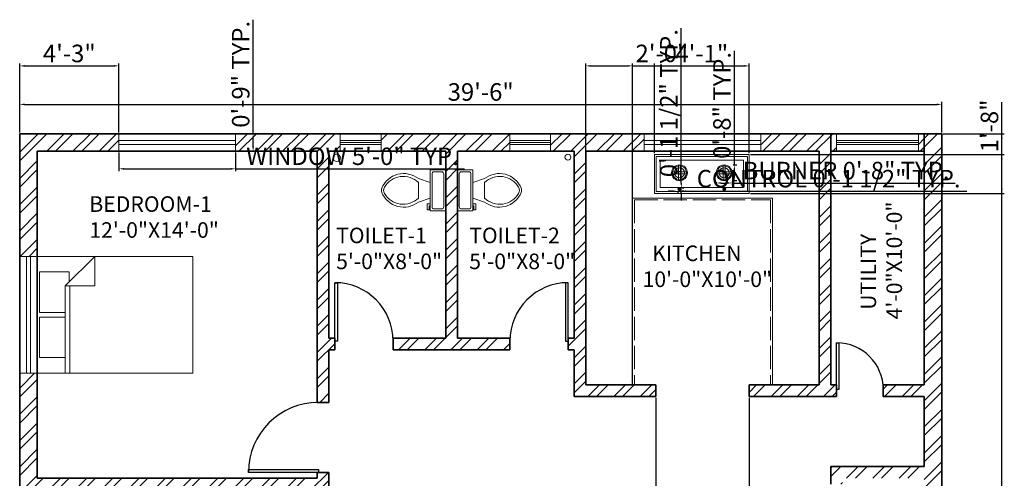
# Model space of a CAD drawing. Units: inches. Extents: x 600 to 1805, y 898 to 2057.
# Tile 3 of 5: x 642 to 1149, y 1822 to 2057. Entities that reach past the tile are written whole.
import ezdxf

# ---------------------------------------------------------------- set-up
doc = ezdxf.new("R2010")
doc.units = ezdxf.units.IN
doc.linetypes.add('ACAD_ISO02W100', pattern=[15, 12, -3])
for name, color, linetype, lineweight in [('A-ANNO-DIMS', 2, 'Continuous', 18), ('A-AREA-IDEN', 7, 'Continuous', 18), ('A-DOOR', 4, 'Continuous', 25), ('A-EQPM', 9, 'Continuous', 18), ('A-FLOR-CASE', 8, 'Continuous', 18), ('A-FLOR-CASE-HIDN', 8, 'ACAD_ISO02W100', 13), ('A-FLOR-FIXT', 8, 'Continuous', 18), ('A-FURN', 8, 'Continuous', 18), ('A-WALL', 7, 'Continuous', 35), ('A-WALL-PATT', 252, 'Continuous', 13)]:
    doc.layers.add(name, color=color, linetype=linetype, lineweight=lineweight)
doc.layers.add('A-GLAZ', color=244, linetype='Continuous', lineweight=20, true_color=0x991b1e)
doc.styles.get("Standard").update_dxf_attribs({"font": 'arial.ttf'})
doc.dimstyles.new('ISO-25', dxfattribs={"dimtxt": 9, "dimasz": 2.5, "dimexe": 1.25, "dimexo": 0.625, "dimtad": 1, "dimlunit": 3, "dimtxsty": 'Standard', "dimcen": 2.5, "dimadec": 0, "dimazin": 0, "dimtfac": 1, "dimtmove": 0, "dimatfit": 3, "dimfxl": 1, "dimarcsym": 0})

# ---------------------------------------------------------------- blocks, each defined once
blk = doc.blocks.new('*U2')
for p, q in [((0, 0), (0, -6)), ((40, 0), (40, -6))]:
    blk.add_line(p, q)
blk.add_lwpolyline([(0, 0), (0, 40), (1.75, 40), (1.75, 0)], close=True)
blk.add_arc((0, 0), 40, 0, 90)
blk = doc.blocks.new('*U3')
for p, q in [((0, 0), (0, -6)), ((-40, 0), (-40, -6))]:
    blk.add_line(p, q)
blk.add_lwpolyline([(0, 0), (0, 40), (-1.75, 40), (-1.75, 0)], close=True)
blk.add_arc((0, 0), 40, 90, 180)
blk = doc.blocks.new('*U4')
for p, q in [((0, 0), (0, -6)), ((40, 0), (40, -6))]:
    blk.add_line(p, q)
blk.add_lwpolyline([(0, 0), (0, 40), (1.75, 40), (1.75, 0)], close=True)
blk.add_arc((0, 0), 40, 0, 90)
blk = doc.blocks.new('Bed - Queen')
for p, q in [((0, -80.00003), (0, 0)), ((0, 0), (59.99999, 0)), ((59.99999, 0), (59.99999, -80.00003)), ((7.99999, -1.2), (28.79998, -1.2)), ((7.99999, -14.4), (7.99999, -1.2)), ((28.79998, -1.2), (28.79998, -14.4)), ((31.19999, -1.2), (51.99999, -1.2)), ((31.19999, -14.4), (31.19999, -1.2)), ((51.99999, -1.2), (51.99999, -16.4)), ((0, -14.4), (44.8, -14.4)), ((59.99999, -29.6), (44.8, -14.4)), ((44.8, -14.4), (44.8, -29.6)), ((44.8, -16.8), (0, -16.8)), ((51.99999, -16.4), (46.79936, -16.4)), ((44.8, -29.6), (59.99999, -29.6)), ((59.99999, -80.00003), (0, -80.00003))]:
    blk.add_line(p, q)
blk = doc.blocks.new('*U10')
for p, q in [((9.5, -6), (9.5, -2)), ((-10, -8.5), (-8, -8.5)), ((-10, -9.5), (-10, -8.5)), ((-7, -9.5), (-10, -9.5)), ((-8, -8.5), (-8, -8)), ((-7, -8), (-7, -9.5)), ((-4, -8), (-6, -14)), ((4, -8), (6, -14)), ((4, -14), (-4, -14))]:
    blk.add_line(p, q)
blk.add_lwpolyline([(10.5, -8), (10.5, 0), (-10.5, 0), (-10.5, -8)], close=True)
for points in [[(-9.5, -2), (-9.5, -6)], [(8.5, -1), (-8.5, -1)], [(-8.5, -7), (8.5, -7)]]:
    blk.add_lwpolyline(points)
for centre, radius, start, end in [((-8.62, -1.88), 0.884, 81.8699, 188.1301), ((8.62, -1.88), 0.884, 351.8699, 98.1301), ((-8.62, -6.12), 0.884, 171.8699, 278.1301), ((8.62, -6.12), 0.884, 261.8699, 8.1301), ((3.52, -21.58), 12.17, 141.4691, 247.9714), ((4.2, -21.82), 11.33, 136.3677, 238.9468), ((-3.52, -21.58), 12.17, 292.0284, 38.5307), ((-4.2, -21.82), 11.33, 301.053, 43.6321), ((0, -27.88), 4, 245.7318, 294.2682), ((0, -29), 4, 254.8605, 285.1395)]:
    blk.add_arc(centre, radius, start, end)
blk = doc.blocks.new('*D13')
at = {"layer": 'A-ANNO-DIMS', "color": 0, "lineweight": -2, "transparency": 16777216}
for p, q in [((642.39, 1999.48), (642.39, 2015.2)), ((1116.39, 1999.48), (1116.39, 2015.2)), ((644.89, 2013.95), (1113.89, 2013.95))]:
    blk.add_line(p, q, dxfattribs=at)
at = {"layer": 'A-ANNO-DIMS', "color": 0, "transparency": 16777216}
for points in [[(644.89, 2014.37), (644.89, 2013.53), (642.39, 2013.95)], [(1113.89, 2014.37), (1113.89, 2013.53), (1116.39, 2013.95)]]:
    blk.add_solid(points, dxfattribs=at)
at = {"layer": 'Defpoints', "color": 0, "transparency": 16777216}
for p in [(1116.39, 2013.95), (642.39, 1998.86), (1116.39, 1998.86)]:
    blk.add_point(p, dxfattribs=at)
at = {"layer": 'A-ANNO-DIMS', "color": 0, "transparency": 16777216, "insert": (879.39, 2019.17), "char_height": 9, "attachment_point": 5}
blk.add_mtext('39\'-6"', dxfattribs=at)
blk = doc.blocks.new('WIN-60x9')
for p, q in [((60, 5.5), (0, 5.5)), ((60, 3.5), (0, 3.5))]:
    blk.add_line(p, q)
blk.add_lwpolyline([(60, 0), (60, 9), (0, 9), (0, 0)], close=True)
blk = doc.blocks.new('VENT-21x9')
for p, q in [((0, 5.5), (21, 5.5)), ((0, 4.5), (21, 4.5)), ((0, 3.5), (21, 3.5))]:
    blk.add_line(p, q)
blk.add_lwpolyline([(21, 9), (21, 0), (0, 0), (0, 9)], close=True)
blk = doc.blocks.new('COOKTOP-BURNER')
for p, q in [((3.54, 8.05), (3.54, 0.03)), ((4.54, 8.05), (4.54, 0.03)), ((0.03, 4.54), (8.05, 4.54)), ((0.03, 3.54), (8.05, 3.54)), ((3.34, 4.74), (3.34, 3.34)), ((3.34, 4.74), (4.74, 4.74)), ((3.34, 3.34), (4.74, 3.34)), ((4.74, 4.74), (4.74, 3.34))]:
    blk.add_line(p, q)
for radius in [4.04, 3.54, 2.54]:
    blk.add_circle((4.04, 4.04), radius)
blk = doc.blocks.new('COOKTOP-CONTROL')
for p, q in [((0, 0.85), (1.49, 0.85)), ((0, 0.65), (1.49, 0.65))]:
    blk.add_line(p, q)
blk.add_circle((0.75, 0.75), 0.747)
for start, end in [(10.5316, 169.4684), (190.5316, 349.4684)]:
    blk.add_arc((0.75, 0.75), 0.547, start, end)
blk = doc.blocks.new('*D22')
at = {"layer": 'A-ANNO-DIMS', "color": 0, "lineweight": -2, "transparency": 16777216}
for p, q in [((693.39, 1989.23), (693.39, 1979.61)), ((753.39, 1989.23), (753.39, 1979.61)), ((695.89, 1980.86), (750.89, 1980.86)), ((753.39, 1980.86), (871.02, 1980.86))]:
    blk.add_line(p, q, dxfattribs=at)
at = {"layer": 'A-ANNO-DIMS', "color": 0, "transparency": 16777216}
for points in [[(695.89, 1981.28), (695.89, 1980.44), (693.39, 1980.86)], [(750.89, 1981.28), (750.89, 1980.44), (753.39, 1980.86)]]:
    blk.add_solid(points, dxfattribs=at)
at = {"layer": 'Defpoints', "color": 0, "transparency": 16777216}
for p in [(693.39, 1989.86), (753.39, 1989.86), (753.39, 1980.86)]:
    blk.add_point(p, dxfattribs=at)
at = {"layer": 'A-ANNO-DIMS', "color": 0, "transparency": 16777216, "insert": (813.46, 1986.14), "char_height": 9, "attachment_point": 5}
blk.add_mtext('WINDOW 5\'-0" TYP.', dxfattribs=at)
blk = doc.blocks.new('*D23')
at = {"layer": 'A-ANNO-DIMS', "color": 0, "lineweight": -2, "transparency": 16777216}
for p, q in [((762.39, 1998.86), (762.39, 2057.47)), ((754.01, 1998.86), (763.64, 1998.86)), ((762.39, 1992.36), (762.39, 1996.36)), ((754.01, 1989.86), (763.64, 1989.86))]:
    blk.add_line(p, q, dxfattribs=at)
at = {"layer": 'A-ANNO-DIMS', "color": 0, "transparency": 16777216}
for points in [[(761.97, 1996.36), (762.8, 1996.36), (762.39, 1998.86)], [(761.97, 1992.36), (762.8, 1992.36), (762.39, 1989.86)]]:
    blk.add_solid(points, dxfattribs=at)
at = {"layer": 'Defpoints', "color": 0, "transparency": 16777216}
for p in [(753.39, 1998.86), (762.39, 1998.86), (753.39, 1989.86)]:
    blk.add_point(p, dxfattribs=at)
at = {"layer": 'A-ANNO-DIMS', "color": 0, "transparency": 16777216, "insert": (757.17, 2029.41), "char_height": 9, "attachment_point": 5, "rotation": 90}
blk.add_mtext('0\'-9" TYP.', dxfattribs=at)
blk = doc.blocks.new('*D28')
at = {"layer": 'A-ANNO-DIMS', "color": 0, "lineweight": -2, "transparency": 16777216}
for p, q in [((1000.52, 1974.15), (1000.52, 1972.32)), ((1003.02, 1973.57), (1006.1, 1973.57)), ((1008.6, 1974.15), (1008.6, 1972.32)), ((1008.6, 1973.57), (1123.4, 1973.57))]:
    blk.add_line(p, q, dxfattribs=at)
at = {"layer": 'A-ANNO-DIMS', "color": 0, "transparency": 16777216}
for points in [[(1003.02, 1973.98), (1003.02, 1973.15), (1000.52, 1973.57)], [(1006.1, 1973.98), (1006.1, 1973.15), (1008.6, 1973.57)]]:
    blk.add_solid(points, dxfattribs=at)
at = {"layer": 'Defpoints', "color": 0, "transparency": 16777216}
for p in [(1000.52, 1974.78), (1008.6, 1974.78), (1008.6, 1973.57)]:
    blk.add_point(p, dxfattribs=at)
at = {"layer": 'A-ANNO-DIMS', "color": 0, "transparency": 16777216, "insert": (1067.25, 1978.79), "char_height": 9, "attachment_point": 5}
blk.add_mtext('BURNER 0\'-8" TYP.', dxfattribs=at)
blk = doc.blocks.new('*D29')
at = {"layer": 'A-ANNO-DIMS', "color": 0, "lineweight": -2, "transparency": 16777216}
for p, q in [((1009.81, 1982.86), (1009.81, 2041.47)), ((1009.23, 1982.86), (1011.06, 1982.86)), ((1009.81, 1977.28), (1009.81, 1980.36)), ((1009.23, 1974.78), (1011.06, 1974.78))]:
    blk.add_line(p, q, dxfattribs=at)
at = {"layer": 'A-ANNO-DIMS', "color": 0, "transparency": 16777216}
for points in [[(1009.4, 1980.36), (1010.23, 1980.36), (1009.81, 1982.86)], [(1009.4, 1977.28), (1010.23, 1977.28), (1009.81, 1974.78)]]:
    blk.add_solid(points, dxfattribs=at)
at = {"layer": 'Defpoints', "color": 0, "transparency": 16777216}
for p in [(1008.6, 1982.86), (1009.81, 1982.86), (1008.6, 1974.78)]:
    blk.add_point(p, dxfattribs=at)
at = {"layer": 'A-ANNO-DIMS', "color": 0, "transparency": 16777216, "insert": (1004.59, 2013.42), "char_height": 9, "attachment_point": 5, "rotation": 90}
blk.add_mtext('0\'-8" TYP.', dxfattribs=at)
blk = doc.blocks.new('*D30')
at = {"layer": 'A-ANNO-DIMS', "color": 0, "lineweight": -2, "transparency": 16777216}
for p, q in [((978.31, 1969.36), (975.81, 1969.36)), ((980.81, 1969.36), (982.3, 1969.36)), ((984.8, 1969.36), (1129.25, 1969.36)), ((980.81, 1968.95), (980.81, 1968.11)), ((982.3, 1968.95), (982.3, 1968.11))]:
    blk.add_line(p, q, dxfattribs=at)
at = {"layer": 'A-ANNO-DIMS', "color": 0, "transparency": 16777216}
for points in [[(978.31, 1969.77), (978.31, 1968.94), (980.81, 1969.36)], [(984.8, 1969.77), (984.8, 1968.94), (982.3, 1969.36)]]:
    blk.add_solid(points, dxfattribs=at)
at = {"layer": 'Defpoints', "color": 0, "transparency": 16777216}
for p in [(980.81, 1969.58), (982.3, 1969.58), (982.3, 1969.36)]:
    blk.add_point(p, dxfattribs=at)
at = {"layer": 'A-ANNO-DIMS', "color": 0, "transparency": 16777216, "insert": (1058.28, 1974.64), "char_height": 9, "attachment_point": 5}
blk.add_mtext('CONTROL 0\'-1 1/2" TYP.', dxfattribs=at)
blk = doc.blocks.new('*D31')
at = {"layer": 'A-ANNO-DIMS', "color": 0, "lineweight": -2, "transparency": 16777216}
for p, q in [((982.53, 1973.57), (982.53, 2053.15)), ((982.53, 1969.58), (982.53, 1971.07)), ((982.93, 1971.07), (983.78, 1971.07)), ((982.93, 1969.58), (983.78, 1969.58)), ((982.53, 1967.08), (982.53, 1964.58))]:
    blk.add_line(p, q, dxfattribs=at)
at = {"layer": 'A-ANNO-DIMS', "color": 0, "transparency": 16777216}
for points in [[(982.11, 1973.57), (982.95, 1973.57), (982.53, 1971.07)], [(982.11, 1967.08), (982.95, 1967.08), (982.53, 1969.58)]]:
    blk.add_solid(points, dxfattribs=at)
at = {"layer": 'Defpoints', "color": 0, "transparency": 16777216}
for p in [(982.3, 1971.07), (982.3, 1969.58), (982.53, 1971.07)]:
    blk.add_point(p, dxfattribs=at)
at = {"layer": 'A-ANNO-DIMS', "color": 0, "transparency": 16777216, "insert": (977.25, 2014.61), "char_height": 9, "attachment_point": 5, "rotation": 90}
blk.add_mtext('0\'-1 1/2" TYP.', dxfattribs=at)
blk = doc.blocks.new('*D32')
at = {"layer": 'A-ANNO-DIMS', "color": 0, "lineweight": -2, "transparency": 16777216}
for p, q in [((1117.01, 1998.86), (1148.59, 1998.86)), ((1147.34, 1455.36), (1147.34, 1996.36)), ((1117.01, 1452.86), (1148.59, 1452.86))]:
    blk.add_line(p, q, dxfattribs=at)
at = {"layer": 'A-ANNO-DIMS', "color": 0, "transparency": 16777216}
for points in [[(1146.92, 1996.36), (1147.75, 1996.36), (1147.34, 1998.86)], [(1146.92, 1455.36), (1147.75, 1455.36), (1147.34, 1452.86)]]:
    blk.add_solid(points, dxfattribs=at)
at = {"layer": 'Defpoints', "color": 0, "transparency": 16777216}
for p in [(1116.39, 1998.86), (1147.34, 1998.86), (1116.39, 1452.86)]:
    blk.add_point(p, dxfattribs=at)
at = {"layer": 'A-ANNO-DIMS', "color": 0, "transparency": 16777216, "insert": (1142.12, 1725.86), "char_height": 9, "attachment_point": 5, "rotation": 90}
blk.add_mtext('45\'-6"', dxfattribs=at)
blk = doc.blocks.new('*D36')
at = {"layer": 'A-ANNO-DIMS', "color": 0, "lineweight": -2, "transparency": 16777216}
for p, q in [((642.39, 1999.48), (642.39, 2035)), ((693.39, 1999.48), (693.39, 2035)), ((644.89, 2033.75), (690.89, 2033.75))]:
    blk.add_line(p, q, dxfattribs=at)
at = {"layer": 'A-ANNO-DIMS', "color": 0, "transparency": 16777216}
for points in [[(644.89, 2034.17), (644.89, 2033.33), (642.39, 2033.75)], [(690.89, 2034.17), (690.89, 2033.33), (693.39, 2033.75)]]:
    blk.add_solid(points, dxfattribs=at)
at = {"layer": 'Defpoints', "color": 0, "transparency": 16777216}
for p in [(693.39, 2033.75), (642.39, 1998.86), (693.39, 1998.86)]:
    blk.add_point(p, dxfattribs=at)
at = {"layer": 'A-ANNO-DIMS', "color": 0, "transparency": 16777216, "insert": (667.89, 2038.97), "char_height": 9, "attachment_point": 5}
blk.add_mtext('4\'-3"', dxfattribs=at)
blk = doc.blocks.new('*D54')
at = {"layer": 'A-ANNO-DIMS', "color": 0, "lineweight": -2, "transparency": 16777216}
for p, q in [((968.67, 1988.87), (968.67, 2035)), ((1017.48, 1988.87), (1017.48, 2035)), ((971.17, 2033.75), (1014.98, 2033.75))]:
    blk.add_line(p, q, dxfattribs=at)
at = {"layer": 'A-ANNO-DIMS', "color": 0, "transparency": 16777216}
for points in [[(971.17, 2034.17), (971.17, 2033.33), (968.67, 2033.75)], [(1014.98, 2034.17), (1014.98, 2033.33), (1017.48, 2033.75)]]:
    blk.add_solid(points, dxfattribs=at)
at = {"layer": 'Defpoints', "color": 0, "transparency": 16777216}
for p in [(1017.48, 2033.75), (968.67, 1988.25), (1017.48, 1988.25)]:
    blk.add_point(p, dxfattribs=at)
at = {"layer": 'A-ANNO-DIMS', "color": 0, "transparency": 16777216, "insert": (993.08, 2038.89), "char_height": 9, "attachment_point": 5}
blk.add_mtext('4\'-1"', dxfattribs=at)
blk = doc.blocks.new('*D55')
at = {"layer": 'A-ANNO-DIMS', "color": 0, "lineweight": -2, "transparency": 16777216}
for p, q in [((1147.34, 1988.25), (1147.34, 2015.07)), ((1018.11, 1988.25), (1148.59, 1988.25)), ((1147.34, 1970.74), (1147.34, 1985.75)), ((1018.11, 1968.24), (1148.59, 1968.24))]:
    blk.add_line(p, q, dxfattribs=at)
at = {"layer": 'A-ANNO-DIMS', "color": 0, "transparency": 16777216}
for points in [[(1146.92, 1985.75), (1147.75, 1985.75), (1147.34, 1988.25)], [(1146.92, 1970.74), (1147.75, 1970.74), (1147.34, 1968.24)]]:
    blk.add_solid(points, dxfattribs=at)
at = {"layer": 'Defpoints', "color": 0, "transparency": 16777216}
for p in [(1017.48, 1988.25), (1147.34, 1988.25), (1017.48, 1968.24)]:
    blk.add_point(p, dxfattribs=at)
at = {"layer": 'A-ANNO-DIMS', "color": 0, "transparency": 16777216, "insert": (1142.12, 2002.91), "char_height": 9, "attachment_point": 5, "rotation": 90}
blk.add_mtext('1\'-8"', dxfattribs=at)
blk = doc.blocks.new('*D56')
at = {"layer": 'A-ANNO-DIMS', "color": 0, "lineweight": -2, "transparency": 16777216}
for p, q in [((933.39, 1870.48), (933.39, 2035)), ((957.39, 1870.48), (957.39, 2035)), ((935.89, 2033.75), (954.89, 2033.75)), ((957.39, 2033.75), (985.21, 2033.75))]:
    blk.add_line(p, q, dxfattribs=at)
at = {"layer": 'A-ANNO-DIMS', "color": 0, "transparency": 16777216}
for points in [[(935.89, 2034.17), (935.89, 2033.33), (933.39, 2033.75)], [(954.89, 2034.17), (954.89, 2033.33), (957.39, 2033.75)]]:
    blk.add_solid(points, dxfattribs=at)
at = {"layer": 'Defpoints', "color": 0, "transparency": 16777216}
for p in [(957.39, 2033.75), (933.39, 1869.86), (957.39, 1869.86)]:
    blk.add_point(p, dxfattribs=at)
at = {"layer": 'A-ANNO-DIMS', "color": 0, "transparency": 16777216, "insert": (972.55, 2038.97), "char_height": 9, "attachment_point": 5}
blk.add_mtext('2\'-0"', dxfattribs=at)
blk = doc.blocks.new('*D57')
at = {"layer": 'A-ANNO-DIMS', "color": 0, "lineweight": -2, "transparency": 16777216}
for p, q in [((969.39, 1863.23), (969.39, 1419.24)), ((1017.39, 1863.23), (1017.39, 1419.24)), ((971.89, 1420.49), (1014.89, 1420.49))]:
    blk.add_line(p, q, dxfattribs=at)
at = {"layer": 'A-ANNO-DIMS', "color": 0, "transparency": 16777216}
for points in [[(971.89, 1420.9), (971.89, 1420.07), (969.39, 1420.49)], [(1014.89, 1420.9), (1014.89, 1420.07), (1017.39, 1420.49)]]:
    blk.add_solid(points, dxfattribs=at)
at = {"layer": 'Defpoints', "color": 0, "transparency": 16777216}
for p in [(969.39, 1863.86), (1017.39, 1863.86), (1017.39, 1420.49)]:
    blk.add_point(p, dxfattribs=at)
at = {"layer": 'A-ANNO-DIMS', "color": 0, "transparency": 16777216, "insert": (993.39, 1425.71), "char_height": 9, "attachment_point": 5}
blk.add_mtext('4\'-0"', dxfattribs=at)

msp = doc.modelspace()

# ---------------------------------------------------------------- hatches: boundary and pattern name
at = {"layer": 'A-WALL-PATT'}
h = msp.add_hatch(dxfattribs=at)
h.set_pattern_fill('ANSI32', color=256)
h.paths.add_polyline_path([(651.387, 1875.859), (642.387, 1875.859), (642.387, 1763.631), (651.387, 1763.631), (651.387, 1815.859), (801.387, 1815.859), (801.387, 1824.859), (795.987, 1824.859), (795.387, 1824.859), (795.387, 1821.859), (651.387, 1821.859)])
h.paths.add_polyline_path([(795.387, 1989.859), (795.387, 1860.859), (801.387, 1860.859), (801.387, 1887.859), (804.387, 1887.859), (804.387, 1892.359), (804.387, 1893.859), (801.387, 1893.859), (801.387, 1989.859), (807.224, 1989.859), (807.224, 1998.859), (753.387, 1998.859), (753.387, 1989.859)])
h.paths.add_polyline_path([(693.387, 1989.859), (693.387, 1998.859), (642.387, 1998.859), (642.387, 1935.859), (651.387, 1935.859), (651.387, 1989.859)])
h.paths.add_polyline_path([(828.224, 1998.859), (828.224, 1989.859), (861.387, 1989.859), (861.387, 1893.859), (834.387, 1893.859), (834.387, 1887.859), (861.387, 1887.859), (894.387, 1887.859), (894.387, 1892.359), (894.387, 1893.859), (867.387, 1893.859), (867.387, 1989.859), (894.316, 1989.859), (894.316, 1998.859)])
h = msp.add_hatch(dxfattribs=at)
h.set_pattern_fill('ANSI32', color=256)
h.paths.add_polyline_path([(933.387, 1989.859), (963.387, 1989.859), (963.387, 1998.859), (915.316, 1998.859), (915.316, 1989.859), (927.387, 1989.859), (927.387, 1893.859), (924.387, 1893.859), (924.387, 1892.359), (924.387, 1887.859), (927.387, 1887.859), (927.387, 1863.859), (969.387, 1863.859), (969.387, 1869.859), (933.387, 1869.859)])
h.paths.add_polyline_path([(1059.387, 1998.859), (1023.387, 1998.859), (1023.387, 1989.859), (1053.387, 1989.859), (1053.387, 1869.859), (1017.387, 1869.859), (1017.387, 1863.859), (1062.387, 1863.859), (1062.387, 1867.459), (1062.387, 1869.859), (1059.387, 1869.859)], flags=17)
h.paths.add_polyline_path([(1116.387, 1998.859), (1107.387, 1998.859), (1107.387, 1869.859), (1086.387, 1869.859), (1086.387, 1863.859), (1107.387, 1863.859), (1107.387, 1827.859), (1059.387, 1827.859), (1059.387, 1818.859), (1065.387, 1818.859), (1065.387, 1821.859), (1107.387, 1821.859), (1107.387, 1667.256), (974.103, 1667.256), (974.103, 1658.256), (1116.387, 1658.256)])
h.paths.add_polyline_path([(953.103, 1667.256), (915.387, 1667.256), (915.387, 1715.256), (882.387, 1715.256), (882.387, 1709.256), (909.387, 1709.256), (909.387, 1637.256), (889.887, 1637.256), (889.887, 1628.256), (915.387, 1628.256), (915.387, 1658.256), (953.103, 1658.256)])
h.paths.add_polyline_path([(868.887, 1637.256), (849.387, 1637.256), (849.387, 1709.256), (852.387, 1709.256), (852.387, 1713.756), (852.387, 1715.256), (849.387, 1715.256), (849.387, 1740.017), (843.387, 1740.017), (843.387, 1647.859), (839.976, 1647.859), (839.976, 1638.859), (843.387, 1638.859), (843.387, 1576.163), (849.387, 1576.163), (849.387, 1628.256), (868.887, 1628.256)])
h.paths.add_polyline_path([(767.566, 1646.059), (767.566, 1647.859), (739.476, 1647.859), (739.476, 1638.859), (767.566, 1638.859)])
h = msp.add_hatch(dxfattribs=at)
h.set_pattern_fill('ANSI32', color=256)
h.paths.add_polyline_path([(1107.387, 1998.859), (1104.387, 1998.859), (1104.387, 1989.859), (1107.387, 1989.859)])
h.paths.add_polyline_path([(1062.387, 1998.859), (1059.387, 1998.859), (1059.387, 1989.859), (1062.387, 1989.859)])

# ---------------------------------------------------------------- linework, layer by layer
at = {"layer": 'A-EQPM'}
for points in [[(968.671, 1988.246), (1017.482, 1988.246), (1017.482, 1968.245), (968.671, 1968.245)], [(969.671, 1987.246), (1016.482, 1987.246), (1016.482, 1969.245), (969.671, 1969.245)], [(971.671, 1985.246), (1014.482, 1985.246), (1014.482, 1971.245), (971.671, 1971.245)]]:
    msp.add_lwpolyline(points, close=True, dxfattribs=at)
at = {"layer": 'A-FLOR-CASE'}
for p, q in [((957.387, 1965.859), (1029.387, 1965.859)), ((957.387, 1965.859), (957.387, 1869.859)), ((1029.387, 1965.859), (1029.387, 1869.859))]:
    msp.add_line(p, q, dxfattribs=at)
at = {"layer": 'A-FLOR-CASE-HIDN'}
for p, q in [((958.387, 1964.859), (1028.387, 1964.859)), ((958.387, 1964.859), (958.387, 1869.859)), ((1028.387, 1964.859), (1028.387, 1869.859))]:
    msp.add_line(p, q, dxfattribs=at)
at = {"layer": 'A-FLOR-FIXT'}
for centre, radius in [((805.404, 1986.492), 1.856), ((924.24, 1986.848), 1.518)]:
    msp.add_circle(centre, radius, dxfattribs=at)
at = {"layer": 'A-GLAZ'}
for p, q in [((1062.387, 1998.859), (1062.387, 1989.859)), ((1062.387, 1995.359), (1104.387, 1995.359)), ((1104.387, 1998.859), (1104.387, 1989.859)), ((1062.387, 1994.359), (1104.387, 1994.359)), ((1062.387, 1993.359), (1104.387, 1993.359))]:
    msp.add_line(p, q, dxfattribs=at)
at = {"layer": 'A-WALL'}
for p, q in [((642.387, 1998.859), (642.387, 1452.859)), ((642.387, 1998.859), (1116.387, 1998.859)), ((1059.387, 1998.859), (1059.387, 1869.859)), ((1107.387, 1998.859), (1107.387, 1869.859)), ((1116.387, 1998.859), (1116.387, 1452.859)), ((651.387, 1989.859), (795.387, 1989.859)), ((651.387, 1989.859), (651.387, 1821.859)), ((795.387, 1989.859), (795.387, 1860.859)), ((801.387, 1989.859), (801.387, 1893.859)), ((801.387, 1989.859), (861.387, 1989.859)), ((861.387, 1989.859), (861.387, 1893.859)), ((867.387, 1989.859), (867.387, 1893.859)), ((867.387, 1989.859), (927.387, 1989.859)), ((927.387, 1989.859), (927.387, 1893.859)), ((933.387, 1989.859), (933.387, 1869.859)), ((933.387, 1989.859), (1053.387, 1989.859)), ((1053.387, 1989.859), (1053.387, 1869.859)), ((1059.387, 1989.859), (1107.387, 1989.859)), ((801.387, 1893.859), (804.387, 1893.859)), ((804.387, 1893.859), (804.387, 1887.859)), ((834.387, 1893.859), (834.387, 1887.859)), ((834.387, 1893.859), (861.387, 1893.859)), ((867.387, 1893.859), (894.387, 1893.859)), ((894.387, 1887.859), (894.387, 1893.859)), ((924.387, 1887.859), (924.387, 1893.859)), ((924.387, 1893.859), (927.387, 1893.859)), ((801.387, 1887.859), (804.387, 1887.859)), ((801.387, 1887.859), (801.387, 1860.859)), ((834.387, 1887.859), (861.387, 1887.859)), ((861.387, 1887.859), (894.387, 1887.859)), ((924.387, 1887.859), (927.387, 1887.859)), ((927.387, 1887.859), (927.387, 1863.859)), ((933.387, 1869.859), (969.387, 1869.859)), ((969.387, 1869.859), (969.387, 1863.859)), ((1017.387, 1869.859), (1017.387, 1863.859)), ((1017.387, 1869.859), (1053.387, 1869.859)), ((1059.387, 1869.859), (1062.387, 1869.859)), ((1062.387, 1869.859), (1062.387, 1863.859)), ((1086.387, 1869.859), (1086.387, 1863.859)), ((1086.387, 1869.859), (1107.387, 1869.859)), ((927.387, 1863.859), (969.387, 1863.859)), ((1017.387, 1863.859), (1062.387, 1863.859)), ((1086.387, 1863.859), (1107.387, 1863.859)), ((1107.387, 1863.859), (1107.387, 1827.859)), ((795.387, 1860.859), (801.387, 1860.859)), ((1059.387, 1827.859), (1107.387, 1827.859)), ((1059.387, 1827.859), (1059.387, 1818.859)), ((795.387, 1824.859), (801.387, 1824.859)), ((795.387, 1824.859), (795.387, 1821.859)), ((801.387, 1824.859), (801.387, 1815.859)), ((651.387, 1821.859), (795.387, 1821.859))]:
    msp.add_line(p, q, dxfattribs=at)

# ---------------------------------------------------------------- block references
at = {"layer": 'A-DOOR'}
for name, p, xscale, yscale, zscale in [('*U2', (804.387, 1892.359), 0.75, 0.75, 0.75), ('*U3', (924.387, 1892.359), 0.75, 0.75, 0.75), ('*U2', (1062.387, 1867.459), 0.6000000000000001, 0.6000000000000001, 0.6000000000000001)]:
    msp.add_blockref(name, p, dxfattribs=dict(at, xscale=xscale, yscale=yscale, zscale=zscale))
at = {"layer": 'A-DOOR', "xscale": 0.9, "yscale": 0.9, "zscale": 0.9, "rotation": 90}
msp.add_blockref('*U4', (795.987, 1824.859), dxfattribs=at)
at = {"layer": 'A-EQPM'}
for name, p in [('COOKTOP-BURNER', (977.553, 1974.78)), ('COOKTOP-BURNER', (1000.515, 1974.78)), ('COOKTOP-CONTROL', (980.811, 1969.58))]:
    msp.add_blockref(name, p, dxfattribs=at)
at = {"layer": 'A-EQPM', "rotation": 180}
msp.add_blockref('COOKTOP-CONTROL', (1005.343, 1971.073), dxfattribs=at)
at = {"layer": 'A-FLOR-FIXT', "xscale": -1, "rotation": 270}
msp.add_blockref('*U10', (861.387, 1969.8), dxfattribs=at)
at = {"layer": 'A-FLOR-FIXT', "rotation": 90}
msp.add_blockref('*U10', (867.387, 1969.8), dxfattribs=at)
at = {"layer": 'A-FURN', "rotation": 90}
msp.add_blockref('Bed - Queen', (651.387, 1875.859), dxfattribs=at)
at = {"layer": 'A-GLAZ'}
for name, p in [('WIN-60x9', (693.387, 1989.859)), ('VENT-21x9', (807.224, 1989.859)), ('VENT-21x9', (894.316, 1989.859)), ('WIN-60x9', (963.387, 1989.859))]:
    msp.add_blockref(name, p, dxfattribs=at)
at = {"layer": 'A-GLAZ', "rotation": 90.00000000000053}
msp.add_blockref('WIN-60x9', (651.386, 1875.859), dxfattribs=at)

# ---------------------------------------------------------------- texts
at = {"layer": 'A-AREA-IDEN', "char_height": 8, "attachment_point": 1}
for s, width, insert in [('BEDROOM-1\\P12\'-0"X14\'-0"', 75.22987, (678.187, 1966.753)), ('TOILET-1\\P5\'-0"X8\'-0"', 51.4853, (805.07, 1950.642)), ('TOILET-2\\P5\'-0"X8\'-0"', 51.4853, (873.493, 1950.642)), ('  KITCHEN\\P10\'-0"X10\'-0"', 63.68907, (962.612, 1941.459))]:
    msp.add_mtext_dynamic_manual_height_columns(s, width=width, gutter_width=12.5, heights=[0], dxfattribs=dict(at, insert=insert))
at = {"layer": 'A-AREA-IDEN', "insert": (1074.659, 1903.523), "char_height": 8, "attachment_point": 1, "rotation": 90}
msp.add_mtext_dynamic_manual_height_columns('  UTILITY\\P4\'-0"X10\'-0"', width=57.59036, gutter_width=12.5, heights=[0], dxfattribs=at)

# ---------------------------------------------------------------- dimensions: what is measured, and where the dimension line sits
at = {"layer": 'A-ANNO-DIMS'}
for base, p1, p2, picture, middle in [((762.387, 1998.859), (753.387, 1989.859), (753.387, 1998.859), '*D23', (757.166, 2029.413)), ((982.529, 1971.074), (982.305, 1969.58), (982.305, 1971.074), '*D31', (977.251, 2014.614)), ((1009.813, 1982.865), (1008.6, 1974.78), (1008.6, 1982.865), '*D29', (1004.593, 2013.42))]:
    dim = msp.add_linear_dim(base=base, p1=p1, p2=p2, angle=90, text='<> TYP.', dimstyle='ISO-25', override={"dimdec": 1, "dimlfac": 1, "dimrnd": 0, "dimzin": 1, "dimdsep": 46, "dimlunit": 4, "dimfrac": 2}, dxfattribs=at)
    dim.commit()
    dim.dimension.update_dxf_attribs({"geometry": picture, "text_midpoint": middle})
for base, p1, p2, override, picture, middle in [((693.387, 2033.75), (642.387, 1998.859), (693.387, 1998.859), {"dimdec": 1, "dimlfac": 1, "dimrnd": 0, "dimzin": 1, "dimdsep": 46, "dimlunit": 4, "dimfrac": 2}, '*D36', (667.887, 2038.973)), ((957.387, 2033.75), (933.387, 1869.859), (957.387, 1869.859), {"dimdec": 1, "dimlfac": 1, "dimrnd": 0, "dimzin": 1, "dimdsep": 46, "dimlunit": 4, "dimfrac": 2}, '*D56', (972.551, 2038.97)), ((1017.482, 2033.75), (968.671, 1988.246), (1017.482, 1988.246), {"dimdec": 1, "dimlfac": 1, "dimrnd": 0, "dimzin": 1, "dimdsep": 46, "dimlunit": 4, "dimfrac": 2}, '*D54', (993.077, 2038.893)), ((1116.387, 2013.951), (642.387, 1998.859), (1116.387, 1998.859), {"dimclrd": 0, "dimclre": 0, "dimclrt": 0}, '*D13', (879.387, 2019.174)), ((1017.387, 1420.485), (969.387, 1863.859), (1017.387, 1863.859), {"dimdec": 1, "dimlfac": 1, "dimrnd": 0, "dimzin": 1, "dimdsep": 46, "dimlunit": 4, "dimfrac": 2}, '*D57', (993.387, 1425.705))]:
    dim = msp.add_linear_dim(base=base, p1=p1, p2=p2, dimstyle='ISO-25', override=override, dxfattribs=at)
    dim.commit()
    dim.dimension.update_dxf_attribs({"geometry": picture, "text_midpoint": middle})
for base, p1, p2, picture, middle in [((1147.337, 1988.246), (1017.482, 1968.245), (1017.482, 1988.246), '*D55', (1142.116, 2002.91)), ((1147.337, 1998.859), (1116.387, 1452.859), (1116.387, 1998.859), '*D32', (1142.116, 1725.859))]:
    dim = msp.add_linear_dim(base=base, p1=p1, p2=p2, angle=90, dimstyle='ISO-25', override={"dimdec": 1, "dimlfac": 1, "dimrnd": 0, "dimzin": 1, "dimdsep": 46, "dimlunit": 4, "dimfrac": 2}, dxfattribs=at)
    dim.commit()
    dim.dimension.update_dxf_attribs({"geometry": picture, "text_midpoint": middle})
for base, p1, p2, text, picture, middle in [((753.387, 1980.859), (693.387, 1989.859), (753.387, 1989.859), 'WINDOW <> TYP.', '*D22', (813.455, 1986.14)), ((982.305, 1969.355), (980.811, 1969.58), (982.305, 1969.58), 'CONTROL <> TYP.', '*D30', (1058.275, 1974.637)), ((1008.6, 1973.567), (1000.515, 1974.78), (1008.6, 1974.78), 'BURNER <> TYP.', '*D28', (1067.248, 1978.787))]:
    dim = msp.add_linear_dim(base=base, p1=p1, p2=p2, text=text, dimstyle='ISO-25', override={"dimdec": 1, "dimlfac": 1, "dimrnd": 0, "dimzin": 1, "dimdsep": 46, "dimlunit": 4, "dimfrac": 2}, dxfattribs=at)
    dim.commit()
    dim.dimension.update_dxf_attribs({"geometry": picture, "text_midpoint": middle})

doc.saveas('drawing.dxf')
